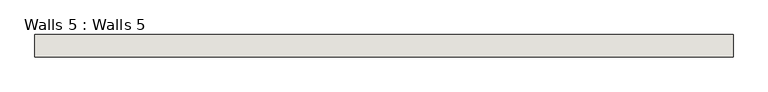
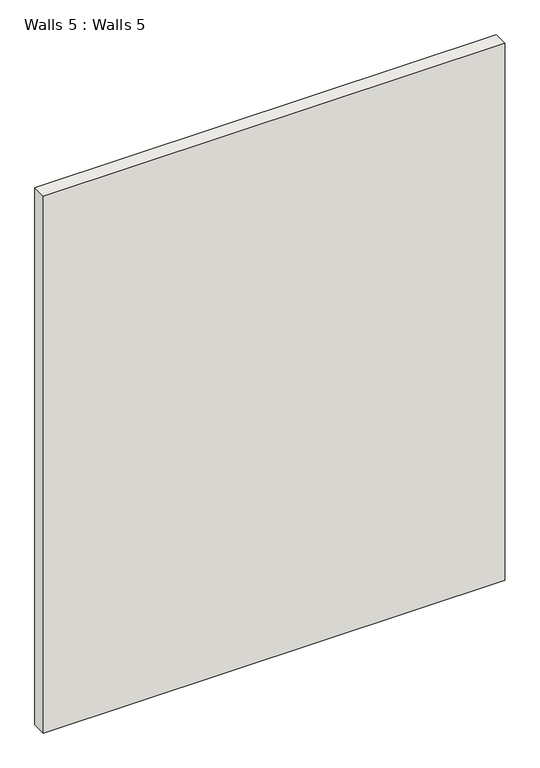
"""IFC4 building model written with IfcOpenShell, lengths in millimetres: wall geometry, Walls 5 : Walls 5."""

from ifc_helpers import new_model, si_unit, frame, origin, place, context, project, spatial, polyline, outline, extrude, source, transform, mapped, element, save


def walls_5_walls_5_5868f2dc(model_context):
    return source(origin(), model_context, "Body", "SweptSolid", [
        extrude(outline(polyline([(-9197.0226654, -7590.0501996), (-12313.0996792, -7590.0501996), (-12313.0996792, -7489.8622642), (-9197.0226654, -7489.8622642), (-9197.0226654, -7590.0501996)])), frame((0.0, 0.0, 2876.6), z_axis=(0.0, 0.0, 1.0), x_axis=(1.0, 0.0, 0.0)), (0.0, 0.0, 1.0), 3833.4962569),
    ])


if __name__ == "__main__":
    model = new_model("IFC4")
    model_context = context("Model", 3, world=origin())
    ifc_project = project(units=[si_unit("LENGTHUNIT", "METRE", prefix="MILLI")], contexts=[model_context])
    site = spatial("IfcSite", under=ifc_project)
    building = spatial("IfcBuilding", under=site)
    placement = place(None, origin())
    walls_5_walls_5_shape = walls_5_walls_5_5868f2dc(model_context)
    element("IfcWall", 1, ObjectType="Walls 5 : Walls 5", at=placement, inside=building, context=model_context, shape_type="MappedRepresentation", body=[
        mapped(walls_5_walls_5_shape, transform((0.0, 0.0, 0.0), x_axis=(1.0, 0.0, 0.0), y_axis=(0.0, 1.0, 0.0), z_axis=(0.0, 0.0, 1.0))),
    ])
    save(model, "model.ifc")

# Revit data of these elements
# Element 1 (IfcWall, "Walls 5 : Walls 5")
#   Materials on its faces: "Default Wall"
# Materials
#   "Default Wall": colour RGB 80 80 80, transparency 0
